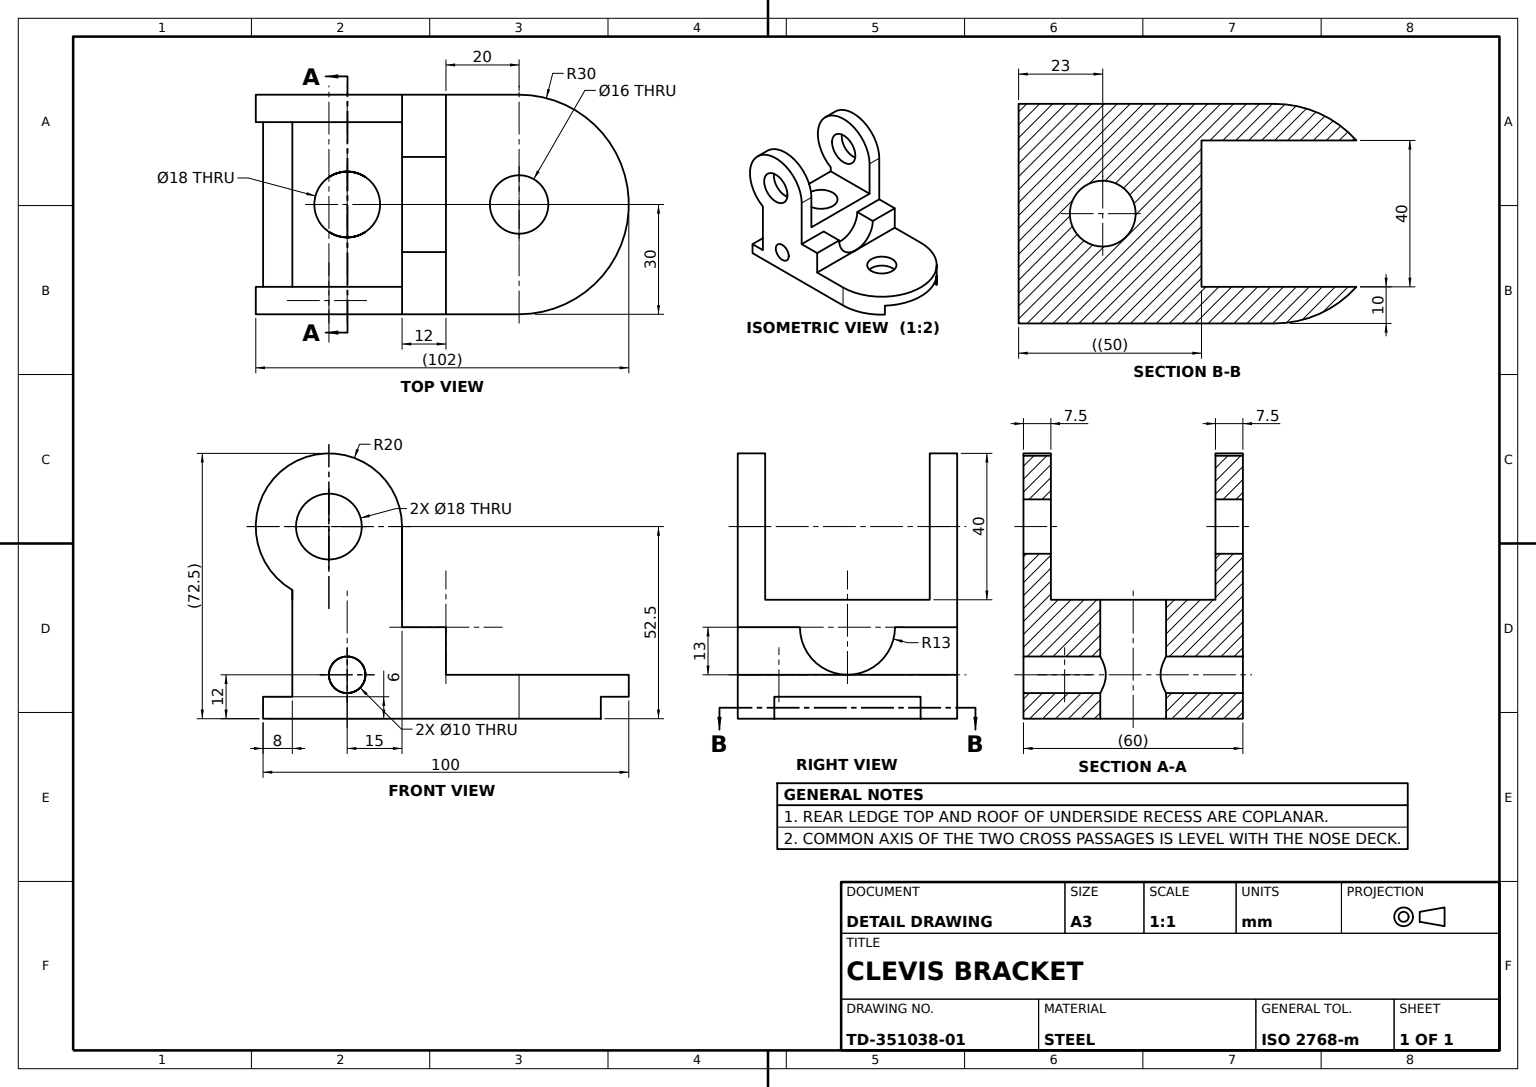
from build123d import *

# Parameters (mm, degrees)
BRACKET_SIDE_PROFILE_SKETCH_R    = 9
BRACKET_SIDE_PROFILE_SKETCH_R_2  = 5
BRACKET_BODY_60MM_DEPTH          = 30
BODY_FILLETS_RADIUS              = 30
BODY_FILLETS_LENGTH              = 12
BORE_13_DEPTH                    = 12
CLEVIS_SLOT_REACH                = 102.001
CLEVIS_SLOT_SKETCH_W             = 45
CLEVIS_SLOT_SKETCH_H             = 40
SADDLE_CUT_REACH                 = 74.139
SADDLE_CUT_SKETCH_R              = 9
SADDLE_CUT_SKETCH_R_2            = 8
BASE_UNDERSIDE_RELIEF_REACH      = 96.129
BASE_UNDERSIDE_RELIEF_END_RADIUS = 30
BASE_UNDERSIDE_RELIEF_SKETCH_W   = 40
BASE_UNDERSIDE_RELIEF_SKETCH_H   = 6


with BuildPart() as part:
    # Bracket Side Profile Sketch → Bracket Body 60mm (new, symmetric)
    with BuildSketch(Plane(origin=(0, 0, 0), x_dir=(0, 0, -1), z_dir=(1, 0, 0))):
        with BuildLine():
            Line((0, 12), (0, 25))
            Line((0, 25), (12, 25))
            Line((12, 25), (12, 52.5))
            ThreePointArc((12, 52.5), (42, 69.820508076), (42, 35.179491924))
            Line((42, 35.179491924), (42, 6))
            Line((42, 6), (50, 6))
            Line((50, 6), (50, 0))
            Line((50, 0), (-50, 0))
            Line((-50, 0), (-50, 12))
            Line((-50, 12), (0, 12))
        make_face()
        with Locations((32, 52.5)):
            Circle(BRACKET_SIDE_PROFILE_SKETCH_R, mode=Mode.SUBTRACT)
        with Locations((27, 12)):
            Circle(BRACKET_SIDE_PROFILE_SKETCH_R_2, mode=Mode.SUBTRACT)
    extrude(amount=BRACKET_BODY_60MM_DEPTH, both=True)

    # Body Fillets: full round fillet: the end face becomes a half cylinder, R = half its width
    body_fillets_face = Plane((0, 6, 50), x_dir=(0, -1, 0), z_dir=(0, 0, 1))  # on the end face: x along it, z out of the body
    body_fillets_slab = body_fillets_face.offset(-BODY_FILLETS_RADIUS / 2) * Box(BODY_FILLETS_LENGTH, 2 * BODY_FILLETS_RADIUS, BODY_FILLETS_RADIUS, mode=Mode.PRIVATE)  # the body's end, R deep
    body_fillets_round = Plane((0, 6, 20), x_dir=(0, 0, 1), z_dir=(0, -1, 0)) * Cylinder(BODY_FILLETS_RADIUS, BODY_FILLETS_LENGTH, mode=Mode.PRIVATE)  # its axis R under the face
    add(body_fillets_slab - body_fillets_round, mode=Mode.SUBTRACT)

    # Bore _13 Sketch → Bore _13 (cut)
    with BuildSketch(Plane.XY):
        with BuildLine():
            Line((-13, 25), (13, 25))
            ThreePointArc((13, 25), (0, 12), (-13, 25))
        make_face()
    extrude(amount=-BORE_13_DEPTH, mode=Mode.SUBTRACT)

    # Clevis Slot Sketch → Clevis Slot (cut, up to next)
    with BuildSketch(Plane.XY.offset(-12), mode=Mode.PRIVATE) as clevis_slot_sk1:
        with Locations((0, 52.5)):
            Rectangle(CLEVIS_SLOT_SKETCH_W, CLEVIS_SLOT_SKETCH_H)
    clevis_slot_tool1 = extrude(clevis_slot_sk1.sketch, amount=-CLEVIS_SLOT_REACH, mode=Mode.PRIVATE) & part.part
    add(clevis_slot_tool1.solids().sort_by_distance((0, 52.5, -12))[0], mode=Mode.SUBTRACT)

    # Saddle Cut: up to this face of the body (flat: up to its plane)
    saddle_cut_end = Plane(part.part.faces().sort_by_distance((0, 0, -2.979428252))[0])
    # Saddle Cut Sketch → Saddle Cut (cut, up to the picked face)
    with BuildSketch(Plane(origin=(0, 32.5, 0), x_dir=(1, 0, 0), z_dir=(0, 1, 0)), mode=Mode.PRIVATE) as saddle_cut_sk1:
        with Locations(Location((0, 27, 0), (0, 0, 180))):
            Circle(SADDLE_CUT_SKETCH_R)
    saddle_cut_tool1 = split(extrude(saddle_cut_sk1.sketch, amount=-SADDLE_CUT_REACH, mode=Mode.PRIVATE), bisect_by=saddle_cut_end, keep=Keep.BOTH, mode=Mode.PRIVATE)
    # Saddle Cut Sketch → Saddle Cut (cut, up to the picked face)
    with BuildSketch(Plane(origin=(0, 32.5, 0), x_dir=(1, 0, 0), z_dir=(0, 1, 0)), mode=Mode.PRIVATE) as saddle_cut_sk2:
        with Locations(Location((0, -20, 0), (0, 0, 270))):
            Circle(SADDLE_CUT_SKETCH_R_2)
    saddle_cut_tool2 = split(extrude(saddle_cut_sk2.sketch, amount=-SADDLE_CUT_REACH, mode=Mode.PRIVATE), bisect_by=saddle_cut_end, keep=Keep.BOTH, mode=Mode.PRIVATE)
    add(saddle_cut_tool1.solids().sort_by(Axis((0, 32.5, -27), (0, -1, 0)))[0], mode=Mode.SUBTRACT)
    add(saddle_cut_tool2.solids().sort_by(Axis((0, 32.5, 20), (0, -1, 0)))[0], mode=Mode.SUBTRACT)

    # Base Underside Relief: up to this cylinder (the profile starts inside it)
    base_underside_relief_end = Plane(origin=(0, 3, 20), z_dir=(0, -1, 0)) * Cylinder(BASE_UNDERSIDE_RELIEF_END_RADIUS, 253.258, mode=Mode.PRIVATE)
    # Base Underside Relief Sketch → Base Underside Relief (cut, up to the surface)
    with BuildSketch(Plane.XY, mode=Mode.PRIVATE) as base_underside_relief_sk1:
        with Locations((0, 3)):
            Rectangle(BASE_UNDERSIDE_RELIEF_SKETCH_W, BASE_UNDERSIDE_RELIEF_SKETCH_H)
    base_underside_relief_tool1 = extrude(base_underside_relief_sk1.sketch, amount=BASE_UNDERSIDE_RELIEF_REACH, mode=Mode.PRIVATE) & base_underside_relief_end
    add(base_underside_relief_tool1.solids().sort_by_distance((0, 3, 0))[0], mode=Mode.SUBTRACT)


solid = part.part
